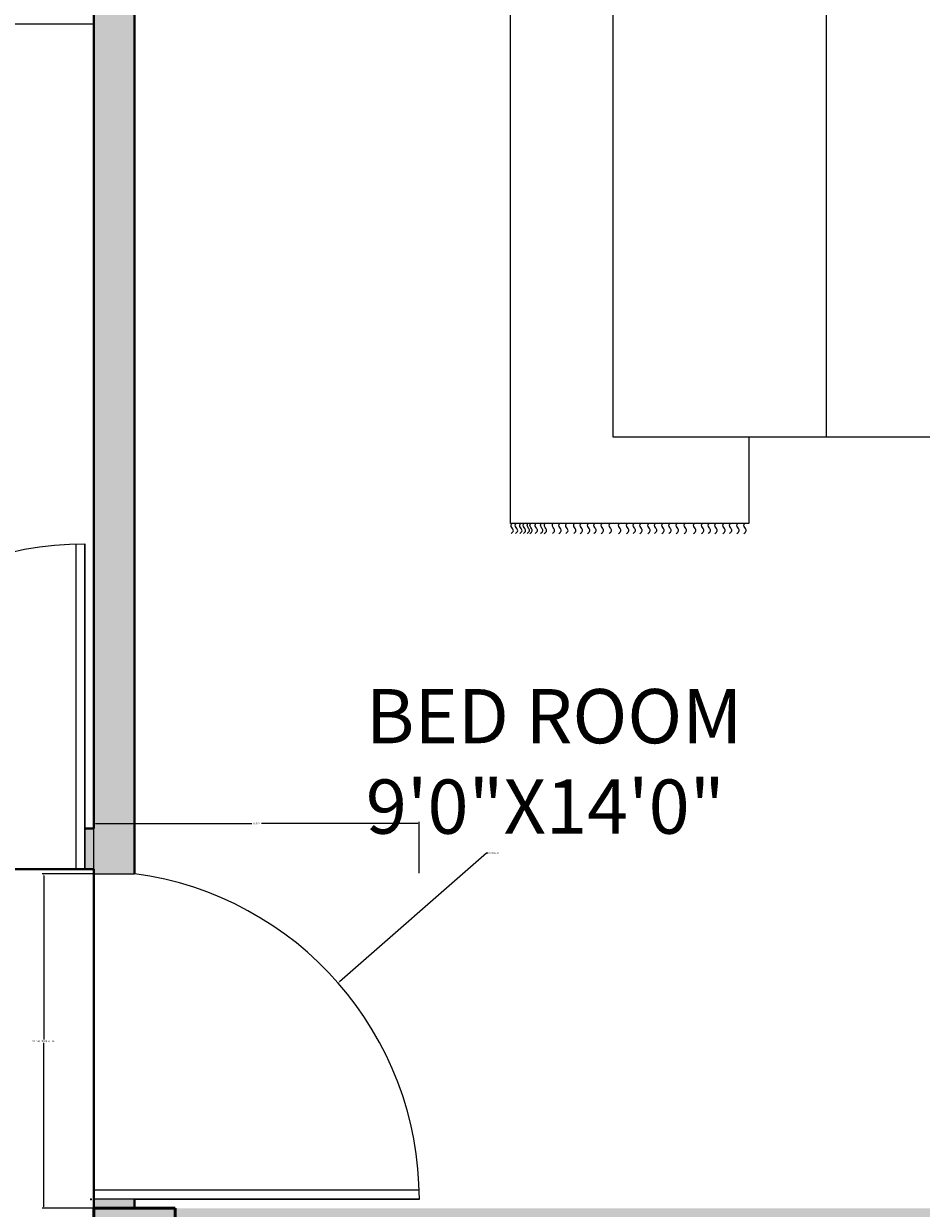
# Model space of a CAD drawing. Units: inches. Extents: x 25176543 to 25177243, y 80295576 to 80296086.
# Tile 8 of 11: x 25176997 to 25177096, y 80295848 to 80295979. Entities that reach past the tile are written whole.
import ezdxf

# ---------------------------------------------------------------- set-up
doc = ezdxf.new("R2010")
doc.units = ezdxf.units.IN
doc.header["$MEASUREMENT"] = 0
for name, color, linetype, lineweight in [('A-ANNO-DIMS', 2, 'Continuous', 18), ('A-AREA-IDEN', 7, 'Continuous', 18), ('A-COLS', 7, 'Continuous', 50), ('A-COLS-PATT', 251, 'Continuous', 13), ('A-DOOR', 3, 'Continuous', 25), ('A-FLOR-CASE', 8, 'Continuous', 25), ('A-WALL', 7, 'Continuous', 40), ('A-WALL-PATT', 146, 'Continuous', 13), ('furniture', 31, 'Continuous', 13)]:
    doc.layers.add(name, color=color, linetype=linetype, lineweight=lineweight)
doc.styles.get("Standard").update_dxf_attribs({"font": 'arial.ttf'})
doc.dimstyles.get("Standard").update_dxf_attribs({"dimtxt": 0.18, "dimasz": 0.18, "dimexe": 0.18, "dimexo": 0.0625, "dimgap": 0.09, "dimtad": 0, "dimtih": 1, "dimtoh": 1, "dimdec": 4, "dimzin": 0, "dimdsep": 46, "dimtxsty": 'Standard', "dimcen": 0.09, "dimadec": 0, "dimazin": 0, "dimtfac": 1, "dimtdec": 4, "dimtofl": 0, "dimtmove": 0, "dimatfit": 3, "dimfxl": 1, "dimtolj": 1, "dimtzin": 0, "dimarcsym": 0})

# ---------------------------------------------------------------- blocks, each defined once
blk = doc.blocks.new('BED-DOUBLE-WITH-NIGHTSTANDS')
for p, q in [((5.6, 61.62), (5.6, 51.56)), ((63.65, 61.72), (63.65, 51.66)), ((10.63, 56.59), (0.57, 56.59)), ((68.68, 56.69), (58.62, 56.69)), ((49.39, 52.82), (10.63, 52.82)), ((49.39, 52.82), (58, 46.47)), ((49.44, 52.82), (49.44, 46.47)), ((49.44, 52), (10.63, 52)), ((49.44, 46.47), (58, 46.47)), ((58.05, 34.96), (10.63, 34.96)), ((4.35, 0), (4.35, 26.37)), ((4.35, 26.37), (10.65, 26.37)), ((58.05, 26.37), (67.59, 26.37)), ((67.59, 26.37), (67.59, 0)), ((67.59, 0), (4.35, 0))]:
    blk.add_line(p, q)
for points in [[(0, 50.39), (10.63, 50.5), (10.63, 62.68), (0, 62.58)], [(58.05, 62.68), (58.05, 11.37), (10.63, 11.37), (10.63, 62.68)], [(58.05, 50.5), (68.68, 50.6), (68.68, 62.78), (58.05, 62.68)], [(29.88, 59.98), (29.88, 52.82), (15.98, 52.82), (15.98, 59.98)], [(49.44, 59.98), (49.44, 52.82), (35.55, 52.82), (35.55, 59.98)]]:
    blk.add_lwpolyline(points, close=True)
for centre in [(5.6, 56.59), (63.65, 56.69)]:
    blk.add_circle(centre, 3.92)
for points, knots in [([(3.23, 25.84), (3.32, 25.96), (3.52, 26.2), (3.86, 25.96), (4.14, 25.78), (4.29, 25.89), (4.35, 25.94)], [0, 0, 0, 0, 0.400747, 0.791423, 1.067667, 1.29709, 1.29709, 1.29709, 1.29709]), ([(3.23, 25.06), (3.32, 25.18), (3.52, 25.42), (3.86, 25.18), (4.14, 25.01), (4.29, 25.11), (4.35, 25.16)], [0, 0, 0, 0, 0.400747, 0.791423, 1.067667, 1.29709, 1.29709, 1.29709, 1.29709]), ([(68.71, 25.84), (68.61, 25.96), (68.42, 26.2), (68.08, 25.96), (67.8, 25.78), (67.65, 25.89), (67.58, 25.94)], [0, 0, 0, 0, 0.400747, 0.791423, 1.067667, 1.29709, 1.29709, 1.29709, 1.29709]), ([(68.71, 25.06), (68.61, 25.18), (68.42, 25.42), (68.08, 25.18), (67.8, 25.01), (67.65, 25.11), (67.58, 25.16)], [0, 0, 0, 0, 0.400747, 0.791423, 1.067667, 1.29709, 1.29709, 1.29709, 1.29709]), ([(3.23, 24.24), (3.32, 24.36), (3.52, 24.6), (3.86, 24.36), (4.14, 24.19), (4.29, 24.3), (4.35, 24.34)], [0, 0, 0, 0, 0.400747, 0.791423, 1.067667, 1.29709, 1.29709, 1.29709, 1.29709]), ([(3.23, 23.51), (3.32, 23.63), (3.52, 23.87), (3.86, 23.63), (4.14, 23.46), (4.29, 23.57), (4.35, 23.62)], [0, 0, 0, 0, 0.400747, 0.791423, 1.067667, 1.29709, 1.29709, 1.29709, 1.29709]), ([(68.71, 24.24), (68.61, 24.36), (68.42, 24.6), (68.08, 24.36), (67.8, 24.19), (67.65, 24.3), (67.58, 24.34)], [0, 0, 0, 0, 0.400747, 0.791423, 1.067667, 1.29709, 1.29709, 1.29709, 1.29709]), ([(68.71, 23.51), (68.61, 23.63), (68.42, 23.87), (68.08, 23.63), (67.8, 23.46), (67.65, 23.57), (67.58, 23.62)], [0, 0, 0, 0, 0.400747, 0.791423, 1.067667, 1.29709, 1.29709, 1.29709, 1.29709]), ([(3.23, 22.63), (3.32, 22.75), (3.52, 22.99), (3.86, 22.75), (4.14, 22.58), (4.29, 22.69), (4.35, 22.73)], [0, 0, 0, 0, 0.400747, 0.791423, 1.067667, 1.29709, 1.29709, 1.29709, 1.29709]), ([(68.71, 22.63), (68.61, 22.75), (68.42, 22.99), (68.08, 22.75), (67.8, 22.58), (67.65, 22.69), (67.58, 22.73)], [0, 0, 0, 0, 0.400747, 0.791423, 1.067667, 1.29709, 1.29709, 1.29709, 1.29709]), ([(3.23, 21.88), (3.32, 22), (3.52, 22.24), (3.86, 22), (4.14, 21.83), (4.29, 21.93), (4.35, 21.98)], [0, 0, 0, 0, 0.400747, 0.791423, 1.067667, 1.29709, 1.29709, 1.29709, 1.29709]), ([(3.23, 21.15), (3.32, 21.27), (3.52, 21.51), (3.86, 21.27), (4.14, 21.1), (4.29, 21.21), (4.35, 21.25)], [0, 0, 0, 0, 0.400747, 0.791423, 1.067667, 1.29709, 1.29709, 1.29709, 1.29709]), ([(68.71, 21.88), (68.61, 22), (68.42, 22.24), (68.08, 22), (67.8, 21.83), (67.65, 21.93), (67.58, 21.98)], [0, 0, 0, 0, 0.400747, 0.791423, 1.067667, 1.29709, 1.29709, 1.29709, 1.29709]), ([(68.71, 21.15), (68.61, 21.27), (68.42, 21.51), (68.08, 21.27), (67.8, 21.1), (67.65, 21.21), (67.58, 21.25)], [0, 0, 0, 0, 0.400747, 0.791423, 1.067667, 1.29709, 1.29709, 1.29709, 1.29709]), ([(3.23, 20.27), (3.32, 20.39), (3.52, 20.63), (3.86, 20.39), (4.14, 20.22), (4.29, 20.32), (4.35, 20.37)], [0, 0, 0, 0, 0.400747, 0.791423, 1.067667, 1.29709, 1.29709, 1.29709, 1.29709]), ([(68.71, 20.27), (68.61, 20.39), (68.42, 20.63), (68.08, 20.39), (67.8, 20.22), (67.65, 20.32), (67.58, 20.37)], [0, 0, 0, 0, 0.400747, 0.791423, 1.067667, 1.29709, 1.29709, 1.29709, 1.29709]), ([(3.23, 19.23), (3.32, 19.35), (3.52, 19.59), (3.86, 19.35), (4.14, 19.18), (4.29, 19.29), (4.35, 19.33)], [0, 0, 0, 0, 0.400747, 0.791423, 1.067667, 1.29709, 1.29709, 1.29709, 1.29709]), ([(3.23, 18.35), (3.32, 18.47), (3.52, 18.71), (3.86, 18.47), (4.14, 18.3), (4.29, 18.4), (4.35, 18.45)], [0, 0, 0, 0, 0.400747, 0.791423, 1.067667, 1.29709, 1.29709, 1.29709, 1.29709]), ([(68.71, 19.23), (68.61, 19.35), (68.42, 19.59), (68.08, 19.35), (67.8, 19.18), (67.65, 19.29), (67.58, 19.33)], [0, 0, 0, 0, 0.400747, 0.791423, 1.067667, 1.29709, 1.29709, 1.29709, 1.29709]), ([(68.71, 18.35), (68.61, 18.47), (68.42, 18.71), (68.08, 18.47), (67.8, 18.3), (67.65, 18.4), (67.58, 18.45)], [0, 0, 0, 0, 0.400747, 0.791423, 1.067667, 1.29709, 1.29709, 1.29709, 1.29709]), ([(3.23, 17.53), (3.32, 17.65), (3.52, 17.89), (3.86, 17.65), (4.14, 17.48), (4.29, 17.59), (4.35, 17.64)], [0, 0, 0, 0, 0.400747, 0.791423, 1.067667, 1.29709, 1.29709, 1.29709, 1.29709]), ([(68.71, 17.53), (68.61, 17.65), (68.42, 17.89), (68.08, 17.65), (67.8, 17.48), (67.65, 17.59), (67.58, 17.64)], [0, 0, 0, 0, 0.400747, 0.791423, 1.067667, 1.29709, 1.29709, 1.29709, 1.29709]), ([(3.23, 16.76), (3.32, 16.88), (3.52, 17.12), (3.86, 16.88), (4.14, 16.7), (4.29, 16.81), (4.35, 16.86)], [0, 0, 0, 0, 0.400747, 0.791423, 1.067667, 1.29709, 1.29709, 1.29709, 1.29709]), ([(3.23, 15.94), (3.32, 16.06), (3.52, 16.3), (3.86, 16.06), (4.14, 15.89), (4.29, 16), (4.35, 16.04)], [0, 0, 0, 0, 0.400747, 0.791423, 1.067667, 1.29709, 1.29709, 1.29709, 1.29709]), ([(68.71, 16.76), (68.61, 16.88), (68.42, 17.12), (68.08, 16.88), (67.8, 16.7), (67.65, 16.81), (67.58, 16.86)], [0, 0, 0, 0, 0.400747, 0.791423, 1.067667, 1.29709, 1.29709, 1.29709, 1.29709]), ([(68.71, 15.94), (68.61, 16.06), (68.42, 16.3), (68.08, 16.06), (67.8, 15.89), (67.65, 16), (67.58, 16.04)], [0, 0, 0, 0, 0.400747, 0.791423, 1.067667, 1.29709, 1.29709, 1.29709, 1.29709]), ([(3.23, 15.21), (3.32, 15.33), (3.52, 15.57), (3.86, 15.33), (4.14, 15.16), (4.29, 15.27), (4.35, 15.32)], [0, 0, 0, 0, 0.400747, 0.791423, 1.067667, 1.29709, 1.29709, 1.29709, 1.29709]), ([(3.23, 14.33), (3.32, 14.45), (3.52, 14.69), (3.86, 14.45), (4.14, 14.28), (4.29, 14.38), (4.35, 14.43)], [0, 0, 0, 0, 0.400747, 0.791423, 1.067667, 1.29709, 1.29709, 1.29709, 1.29709]), ([(68.71, 15.21), (68.61, 15.33), (68.42, 15.57), (68.08, 15.33), (67.8, 15.16), (67.65, 15.27), (67.58, 15.32)], [0, 0, 0, 0, 0.400747, 0.791423, 1.067667, 1.29709, 1.29709, 1.29709, 1.29709]), ([(68.71, 14.33), (68.61, 14.45), (68.42, 14.69), (68.08, 14.45), (67.8, 14.28), (67.65, 14.38), (67.58, 14.43)], [0, 0, 0, 0, 0.400747, 0.791423, 1.067667, 1.29709, 1.29709, 1.29709, 1.29709]), ([(3.23, 13.58), (3.32, 13.7), (3.52, 13.94), (3.86, 13.7), (4.14, 13.53), (4.29, 13.63), (4.35, 13.68)], [0, 0, 0, 0, 0.400747, 0.791423, 1.067667, 1.29709, 1.29709, 1.29709, 1.29709]), ([(3.23, 12.85), (3.32, 12.97), (3.52, 13.21), (3.86, 12.97), (4.14, 12.8), (4.29, 12.9), (4.35, 12.95)], [0, 0, 0, 0, 0.400747, 0.791423, 1.067667, 1.29709, 1.29709, 1.29709, 1.29709]), ([(68.71, 13.58), (68.61, 13.7), (68.42, 13.94), (68.08, 13.7), (67.8, 13.53), (67.65, 13.63), (67.58, 13.68)], [0, 0, 0, 0, 0.400747, 0.791423, 1.067667, 1.29709, 1.29709, 1.29709, 1.29709]), ([(68.71, 12.85), (68.61, 12.97), (68.42, 13.21), (68.08, 12.97), (67.8, 12.8), (67.65, 12.9), (67.58, 12.95)], [0, 0, 0, 0, 0.400747, 0.791423, 1.067667, 1.29709, 1.29709, 1.29709, 1.29709]), ([(3.23, 11.97), (3.32, 12.09), (3.52, 12.33), (3.86, 12.09), (4.14, 11.92), (4.29, 12.02), (4.35, 12.07)], [0, 0, 0, 0, 0.400747, 0.791423, 1.067667, 1.29709, 1.29709, 1.29709, 1.29709]), ([(68.71, 11.97), (68.61, 12.09), (68.42, 12.33), (68.08, 12.09), (67.8, 11.92), (67.65, 12.02), (67.58, 12.07)], [0, 0, 0, 0, 0.400747, 0.791423, 1.067667, 1.29709, 1.29709, 1.29709, 1.29709]), ([(3.23, 10.93), (3.32, 11.05), (3.52, 11.29), (3.86, 11.05), (4.14, 10.88), (4.29, 10.99), (4.35, 11.03)], [0, 0, 0, 0, 0.400747, 0.791423, 1.067667, 1.29709, 1.29709, 1.29709, 1.29709]), ([(68.71, 10.93), (68.61, 11.05), (68.42, 11.29), (68.08, 11.05), (67.8, 10.88), (67.65, 10.99), (67.58, 11.03)], [0, 0, 0, 0, 0.400747, 0.791423, 1.067667, 1.29709, 1.29709, 1.29709, 1.29709]), ([(3.23, 10.05), (3.32, 10.17), (3.52, 10.41), (3.86, 10.17), (4.14, 10), (4.29, 10.1), (4.35, 10.15)], [0, 0, 0, 0, 0.400747, 0.791423, 1.067667, 1.29709, 1.29709, 1.29709, 1.29709]), ([(3.23, 9.23), (3.32, 9.35), (3.52, 9.59), (3.86, 9.35), (4.14, 9.18), (4.29, 9.29), (4.35, 9.34)], [0, 0, 0, 0, 0.400747, 0.791423, 1.067667, 1.29709, 1.29709, 1.29709, 1.29709]), ([(68.71, 10.05), (68.61, 10.17), (68.42, 10.41), (68.08, 10.17), (67.8, 10), (67.65, 10.1), (67.58, 10.15)], [0, 0, 0, 0, 0.400747, 0.791423, 1.067667, 1.29709, 1.29709, 1.29709, 1.29709]), ([(68.71, 9.23), (68.61, 9.35), (68.42, 9.59), (68.08, 9.35), (67.8, 9.18), (67.65, 9.29), (67.58, 9.34)], [0, 0, 0, 0, 0.400747, 0.791423, 1.067667, 1.29709, 1.29709, 1.29709, 1.29709]), ([(3.23, 8.54), (3.32, 8.66), (3.52, 8.9), (3.86, 8.66), (4.14, 8.49), (4.29, 8.6), (4.35, 8.65)], [0, 0, 0, 0, 0.400747, 0.791423, 1.067667, 1.29709, 1.29709, 1.29709, 1.29709]), ([(3.23, 7.73), (3.32, 7.85), (3.52, 8.09), (3.86, 7.85), (4.14, 7.68), (4.29, 7.78), (4.35, 7.83)], [0, 0, 0, 0, 0.400747, 0.791423, 1.067667, 1.29709, 1.29709, 1.29709, 1.29709]), ([(68.71, 8.54), (68.61, 8.66), (68.42, 8.9), (68.08, 8.66), (67.8, 8.49), (67.65, 8.6), (67.58, 8.65)], [0, 0, 0, 0, 0.400747, 0.791423, 1.067667, 1.29709, 1.29709, 1.29709, 1.29709]), ([(68.71, 7.73), (68.61, 7.85), (68.42, 8.09), (68.08, 7.85), (67.8, 7.68), (67.65, 7.78), (67.58, 7.83)], [0, 0, 0, 0, 0.400747, 0.791423, 1.067667, 1.29709, 1.29709, 1.29709, 1.29709]), ([(3.23, 7), (3.32, 7.12), (3.52, 7.36), (3.86, 7.12), (4.14, 6.95), (4.29, 7.05), (4.35, 7.1)], [0, 0, 0, 0, 0.400747, 0.791423, 1.067667, 1.29709, 1.29709, 1.29709, 1.29709]), ([(68.71, 7), (68.61, 7.12), (68.42, 7.36), (68.08, 7.12), (67.8, 6.95), (67.65, 7.05), (67.58, 7.1)], [0, 0, 0, 0, 0.400747, 0.791423, 1.067667, 1.29709, 1.29709, 1.29709, 1.29709]), ([(3.23, 6.12), (3.32, 6.24), (3.52, 6.48), (3.86, 6.24), (4.14, 6.07), (4.29, 6.17), (4.35, 6.22)], [0, 0, 0, 0, 0.400747, 0.791423, 1.067667, 1.29709, 1.29709, 1.29709, 1.29709]), ([(3.23, 5.36), (3.32, 5.49), (3.52, 5.73), (3.86, 5.49), (4.14, 5.31), (4.29, 5.42), (4.35, 5.47)], [0, 0, 0, 0, 0.400747, 0.791423, 1.067667, 1.29709, 1.29709, 1.29709, 1.29709]), ([(68.71, 6.12), (68.61, 6.24), (68.42, 6.48), (68.08, 6.24), (67.8, 6.07), (67.65, 6.17), (67.58, 6.22)], [0, 0, 0, 0, 0.400747, 0.791423, 1.067667, 1.29709, 1.29709, 1.29709, 1.29709]), ([(68.71, 5.36), (68.61, 5.49), (68.42, 5.73), (68.08, 5.49), (67.8, 5.31), (67.65, 5.42), (67.58, 5.47)], [0, 0, 0, 0, 0.400747, 0.791423, 1.067667, 1.29709, 1.29709, 1.29709, 1.29709]), ([(3.23, 4.64), (3.32, 4.76), (3.52, 5), (3.86, 4.76), (4.14, 4.59), (4.29, 4.69), (4.35, 4.74)], [0, 0, 0, 0, 0.400747, 0.791423, 1.067667, 1.29709, 1.29709, 1.29709, 1.29709]), ([(3.23, 3.75), (3.32, 3.88), (3.52, 4.12), (3.86, 3.88), (4.14, 3.7), (4.29, 3.81), (4.35, 3.86)], [0, 0, 0, 0, 0.400747, 0.791423, 1.067667, 1.29709, 1.29709, 1.29709, 1.29709]), ([(68.71, 4.64), (68.61, 4.76), (68.42, 5), (68.08, 4.76), (67.8, 4.59), (67.66, 4.69), (67.59, 4.73)], [0, 0, 0, 0, 0.400747, 0.791423, 1.067667, 1.283686, 1.283686, 1.283686, 1.283686]), ([(68.71, 3.75), (68.61, 3.88), (68.42, 4.11), (68.08, 3.88), (67.8, 3.7), (67.66, 3.81), (67.59, 3.85)], [0, 0, 0, 0, 0.400747, 0.791423, 1.067667, 1.283686, 1.283686, 1.283686, 1.283686]), ([(3.23, 3.33), (3.32, 3.45), (3.52, 3.7), (3.86, 3.44), (4.14, 3.27), (4.29, 3.38), (4.35, 3.43)], [0, 0, 0, 0, 0.407265, 0.802015, 1.07826, 1.307683, 1.307683, 1.307683, 1.307683]), ([(3.23, 2.76), (3.32, 2.88), (3.52, 3.12), (3.86, 2.88), (4.14, 2.71), (4.29, 2.81), (4.35, 2.86)], [0, 0, 0, 0, 0.400747, 0.791423, 1.067667, 1.29709, 1.29709, 1.29709, 1.29709]), ([(68.71, 3.33), (68.61, 3.45), (68.42, 3.69), (68.08, 3.45), (67.8, 3.27), (67.66, 3.38), (67.59, 3.42)], [0, 0, 0, 0, 0.402903, 0.794912, 1.071156, 1.287177, 1.287177, 1.287177, 1.287177]), ([(68.71, 2.73), (68.61, 2.85), (68.42, 3.09), (68.08, 2.85), (67.8, 2.68), (67.66, 2.78), (67.59, 2.82)], [0, 0, 0, 0, 0.400747, 0.791423, 1.067667, 1.283686, 1.283686, 1.283686, 1.283686]), ([(3.23, 2.18), (3.32, 2.31), (3.52, 2.55), (3.86, 2.31), (4.14, 2.13), (4.29, 2.24), (4.35, 2.29)], [0, 0, 0, 0, 0.400747, 0.791423, 1.067667, 1.29709, 1.29709, 1.29709, 1.29709]), ([(3.23, 1.88), (3.32, 2), (3.52, 2.24), (3.86, 2), (4.14, 1.82), (4.29, 1.93), (4.35, 1.98)], [0, 0, 0, 0, 0.400747, 0.791423, 1.067667, 1.29709, 1.29709, 1.29709, 1.29709]), ([(3.23, 1.46), (3.32, 1.58), (3.52, 1.82), (3.86, 1.58), (4.14, 1.41), (4.29, 1.51), (4.35, 1.56)], [0, 0, 0, 0, 0.400747, 0.791423, 1.067667, 1.29709, 1.29709, 1.29709, 1.29709]), ([(3.23, 1.06), (3.32, 1.18), (3.52, 1.42), (3.86, 1.18), (4.14, 1.01), (4.29, 1.11), (4.35, 1.16)], [0, 0, 0, 0, 0.400747, 0.791423, 1.067667, 1.29709, 1.29709, 1.29709, 1.29709]), ([(68.71, 1.43), (68.61, 1.55), (68.42, 1.79), (68.08, 1.55), (67.8, 1.38), (67.65, 1.48), (67.58, 1.53)], [0, 0, 0, 0, 0.400747, 0.791423, 1.067667, 1.29709, 1.29709, 1.29709, 1.29709]), ([(68.71, 2.16), (68.61, 2.28), (68.42, 2.52), (68.08, 2.28), (67.8, 2.11), (67.66, 2.21), (67.59, 2.25)], [0, 0, 0, 0, 0.400747, 0.791423, 1.067667, 1.283686, 1.283686, 1.283686, 1.283686]), ([(68.71, 1.85), (68.61, 1.97), (68.42, 2.21), (68.08, 1.97), (67.8, 1.8), (67.66, 1.9), (67.59, 1.94)], [0, 0, 0, 0, 0.400747, 0.791423, 1.067667, 1.283686, 1.283686, 1.283686, 1.283686]), ([(3.23, 0.57), (3.32, 0.7), (3.52, 0.94), (3.86, 0.7), (4.14, 0.52), (4.29, 0.63), (4.35, 0.68)], [0, 0, 0, 0, 0.400747, 0.791423, 1.067667, 1.29709, 1.29709, 1.29709, 1.29709]), ([(3.23, 0.07), (3.32, 0.19), (3.52, 0.43), (3.86, 0.19), (4.14, 0.02), (4.29, 0.13), (4.35, 0.18)], [0, 0, 0, 0, 0.400747, 0.791423, 1.067667, 1.29709, 1.29709, 1.29709, 1.29709]), ([(68.71, 1.03), (68.61, 1.15), (68.42, 1.39), (68.08, 1.15), (67.8, 0.98), (67.65, 1.09), (67.58, 1.13)], [0, 0, 0, 0, 0.400747, 0.791423, 1.067667, 1.29709, 1.29709, 1.29709, 1.29709]), ([(68.71, 0.55), (68.61, 0.67), (68.42, 0.91), (68.08, 0.67), (67.8, 0.49), (67.65, 0.6), (67.58, 0.65)], [0, 0, 0, 0, 0.400747, 0.791423, 1.067667, 1.29709, 1.29709, 1.29709, 1.29709]), ([(68.71, 0.07), (68.61, 0.19), (68.42, 0.43), (68.08, 0.19), (67.8, 0.02), (67.65, 0.13), (67.58, 0.18)], [0, 0, 0, 0, 0.400747, 0.791423, 1.067667, 1.29709, 1.29709, 1.29709, 1.29709])]:
    blk.add_open_spline(points, degree=3, knots=knots)
blk = doc.blocks.new('DOOR-36IN')
for p, q in [((36, 37), (31.5, 37)), ((36, 1), (36, 37)), ((0, 2), (36, 2)), ((36, 1), (0, 1)), ((0, 1), (36, 1)), ((36, 0), (36, 1))]:
    blk.add_line(p, q)
blk.add_arc((36.32, 1), 36.32, 97.6281, 180)
blk = doc.blocks.new('DOOR-36IN-OFFSET')
for p, q in [((0, 1), (0, 37)), ((0, 37), (4.5, 37)), ((36, 2), (0, 2)), ((0, 0), (0, 1)), ((4.5, 1), (0, 1)), ((4.5, 1), (36, 1)), ((36, 1), (4.5, 1))]:
    blk.add_line(p, q)
blk.add_arc((-0.32, 1), 36.32, 0, 82.3719)
blk = doc.blocks.new('COLUMN-9IN-SQ')
for p, q in [((9, 9), (0, 9)), ((0, 9), (0, 0)), ((9, 0), (9, 9)), ((0, 0), (9, 0))]:
    blk.add_line(p, q)
blk = doc.blocks.new('*D42')
at = {"layer": 'A-ANNO-DIMS', "color": 0, "lineweight": -2, "transparency": 16777216}
for p, q in [((25177004.24, 80295885.3), (25176998.57, 80295885.3)), ((25176998.75, 80295885.12), (25176998.75, 80295866.99)), ((25176998.75, 80295848.48), (25176998.75, 80295866.62)), ((25177004.24, 80295848.3), (25176998.57, 80295848.3))]:
    blk.add_line(p, q, dxfattribs=at)
at = {"layer": 'A-ANNO-DIMS', "color": 0, "transparency": 16777216}
for points in [[(25176998.72, 80295885.12), (25176998.78, 80295885.12), (25176998.75, 80295885.3)], [(25176998.72, 80295848.48), (25176998.78, 80295848.48), (25176998.75, 80295848.3)]]:
    blk.add_solid(points, dxfattribs=at)
at = {"layer": 'Defpoints', "color": 0, "transparency": 16777216}
for p in [(25176998.75, 80295885.3), (25177004.3, 80295885.3), (25177004.3, 80295848.3)]:
    blk.add_point(p, dxfattribs=at)
at = {"layer": 'A-ANNO-DIMS', "color": 0, "transparency": 16777216, "insert": (25176998.75, 80295866.8), "char_height": 0.18, "attachment_point": 5}
blk.add_mtext('\\A1;OFFSET DOOR 37 TYP.', dxfattribs=at)
blk = doc.blocks.new('*D43')
at = {"layer": 'A-ANNO-DIMS', "color": 0, "lineweight": -2, "transparency": 16777216}
for p, q in [((25177004.3, 80295885.36), (25177004.3, 80295891.03)), ((25177004.48, 80295890.85), (25177021.77, 80295890.85)), ((25177040.12, 80295890.85), (25177022.83, 80295890.85)), ((25177040.3, 80295885.36), (25177040.3, 80295891.03))]:
    blk.add_line(p, q, dxfattribs=at)
at = {"layer": 'A-ANNO-DIMS', "color": 0, "transparency": 16777216}
for points in [[(25177004.48, 80295890.88), (25177004.48, 80295890.82), (25177004.3, 80295890.85)], [(25177040.12, 80295890.88), (25177040.12, 80295890.82), (25177040.3, 80295890.85)]]:
    blk.add_solid(points, dxfattribs=at)
at = {"layer": 'Defpoints', "color": 0, "transparency": 16777216}
for p in [(25177040.3, 80295890.85), (25177004.3, 80295885.3), (25177040.3, 80295885.3)]:
    blk.add_point(p, dxfattribs=at)
at = {"layer": 'A-ANNO-DIMS', "color": 0, "transparency": 16777216, "insert": (25177022.3, 80295890.85), "char_height": 0.18, "attachment_point": 5}
blk.add_mtext('\\A1;36 TYP.', dxfattribs=at)
blk = doc.blocks.new('*D48')
at = {"layer": 'A-ANNO-DIMS', "color": 0, "lineweight": -2, "transparency": 16777216}
for p, q in [((25176625.3, 80295890.36), (25176625.3, 80296052.23)), ((25176625.48, 80296052.05), (25176875.16, 80296052.05)), ((25177125.62, 80296052.05), (25176875.95, 80296052.05)), ((25177125.8, 80296025.36), (25177125.8, 80296052.23))]:
    blk.add_line(p, q, dxfattribs=at)
at = {"layer": 'A-ANNO-DIMS', "color": 0, "transparency": 16777216}
for points in [[(25176625.48, 80296052.08), (25176625.48, 80296052.02), (25176625.3, 80296052.05)], [(25177125.62, 80296052.08), (25177125.62, 80296052.02), (25177125.8, 80296052.05)]]:
    blk.add_solid(points, dxfattribs=at)
at = {"layer": 'Defpoints', "color": 0, "transparency": 16777216}
for p in [(25177125.8, 80296052.05), (25177125.8, 80296025.3), (25176625.3, 80295890.3)]:
    blk.add_point(p, dxfattribs=at)
at = {"layer": 'A-ANNO-DIMS', "color": 0, "transparency": 16777216, "insert": (25176875.55, 80296052.05), "char_height": 0.18, "attachment_point": 5}
blk.add_mtext('\\A1;500.5', dxfattribs=at)
blk = doc.blocks.new('*D76')
at = {"layer": 'A-ANNO-DIMS', "color": 0, "lineweight": -2, "transparency": 16777216}
for p, q in [((25177047.72, 80295887.57), (25177031.45, 80295873.34)), ((25177047.9, 80295887.57), (25177047.72, 80295887.57)), ((25177003.89, 80295849.3), (25177004.07, 80295849.3)), ((25177003.98, 80295849.21), (25177003.98, 80295849.39))]:
    blk.add_line(p, q, dxfattribs=at)
at = {"layer": 'A-ANNO-DIMS', "color": 0, "transparency": 16777216}
blk.add_solid([(25177031.43, 80295873.36), (25177031.47, 80295873.32), (25177031.31, 80295873.22)], dxfattribs=at)
at = {"layer": 'Defpoints', "color": 0, "transparency": 16777216}
for p in [(25177031.31, 80295873.22), (25177003.98, 80295849.3)]:
    blk.add_point(p, dxfattribs=at)
at = {"layer": 'A-ANNO-DIMS', "color": 0, "transparency": 16777216, "insert": (25177048.57, 80295887.57), "char_height": 0.18, "attachment_point": 5}
blk.add_mtext('\\A1;2X R36.32', dxfattribs=at)

msp = doc.modelspace()

# ---------------------------------------------------------------- hatches: boundary and pattern name
at = {"layer": 'A-COLS-PATT'}
h = msp.add_hatch(color=256, dxfattribs=at)
h.dxf.hatch_style = 1
h.paths.add_polyline_path([(25176658.8016, 80296025.3022), (25176649.8016, 80296025.3022), (25176649.8016, 80296016.3022), (25176658.8016, 80296016.3022)])
h.paths.add_polyline_path([(25176819.3016, 80296025.3022), (25176810.3016, 80296025.3022), (25176810.3016, 80296016.3022), (25176819.3016, 80296016.3022)])
h.paths.add_polyline_path([(25176876.3016, 80296025.3022), (25176867.3016, 80296025.3022), (25176867.3016, 80296016.3022), (25176876.3016, 80296016.3022)])
h.paths.add_polyline_path([(25177013.3016, 80296025.3022), (25177004.3016, 80296025.3022), (25177004.3016, 80296016.3022), (25177013.3016, 80296016.3022)])
h.paths.add_polyline_path([(25176819.3016, 80295890.3022), (25176810.3016, 80295890.3022), (25176810.3016, 80295881.3022), (25176819.3016, 80295881.3022)])
h.paths.add_polyline_path([(25176658.8016, 80295890.3022), (25176649.8016, 80295890.3022), (25176649.8016, 80295881.3022), (25176658.8016, 80295881.3022)])
h.paths.add_polyline_path([(25177125.8016, 80296025.3022), (25177116.8016, 80296025.3022), (25177116.8016, 80296016.3022), (25177125.8016, 80296016.3022)])
h.paths.add_polyline_path([(25177125.8016, 80295848.3022), (25177116.8016, 80295848.3022), (25177116.8016, 80295839.3022), (25177125.8016, 80295839.3022)])
h.paths.add_polyline_path([(25177013.3016, 80295848.3022), (25177004.3016, 80295848.3022), (25177004.3016, 80295839.3022), (25177013.3016, 80295839.3022)])
h.paths.add_polyline_path([(25177125.8016, 80295676.8022), (25177116.8016, 80295676.8022), (25177116.8016, 80295667.8022), (25177125.8016, 80295667.8022)])
h.paths.add_polyline_path([(25177013.3016, 80295676.8022), (25177004.3016, 80295676.8022), (25177004.3016, 80295667.8022), (25177013.3016, 80295667.8022)])
h.paths.add_polyline_path([(25176842.3016, 80295676.8022), (25176833.3016, 80295676.8022), (25176833.3016, 80295667.8022), (25176842.3016, 80295667.8022)])
h.paths.add_polyline_path([(25176893.3016, 80295676.8022), (25176884.3016, 80295676.8022), (25176884.3016, 80295667.8022), (25176893.3016, 80295667.8022)])
h.paths.add_polyline_path([(25176842.3016, 80295807.3022), (25176833.3016, 80295807.3022), (25176833.3016, 80295798.3022), (25176842.3016, 80295798.3022)])
h.paths.add_polyline_path([(25176658.8016, 80295807.3022), (25176649.8016, 80295807.3022), (25176649.8016, 80295798.3022), (25176658.8016, 80295798.3022)])
h.paths.add_polyline_path([(25176658.8016, 80295676.8022), (25176649.8016, 80295676.8022), (25176649.8016, 80295667.8022), (25176658.8016, 80295667.8022)])
at = {"layer": 'A-WALL-PATT'}
h = msp.add_hatch(color=256, dxfattribs=at)
h.dxf.hatch_style = 1
h.paths.add_polyline_path([(25176695.189, 80296025.3022), (25176658.8016, 80296025.3022), (25176658.8016, 80296016.3022), (25176695.189, 80296016.3022)])
h.paths.add_polyline_path([(25176810.3016, 80296025.3022), (25176755.189, 80296025.3022), (25176755.189, 80296016.3022), (25176810.3016, 80296016.3022)])
h.paths.add_polyline_path([(25176819.3016, 80296016.3022), (25176814.8016, 80296016.3022), (25176814.8016, 80295965.3022), (25176819.3016, 80295965.3022)], flags=17)
h.paths.add_polyline_path([(25176828.0421, 80296025.3022), (25176819.3016, 80296025.3022), (25176819.3016, 80296016.3022), (25176828.0421, 80296016.3022)])
h.paths.add_polyline_path([(25176867.3016, 80296025.3022), (25176852.0421, 80296025.3022), (25176852.0421, 80296016.3022), (25176867.3016, 80296016.3022)])
h.paths.add_polyline_path([(25176885.1873, 80296025.3022), (25176876.3016, 80296025.3022), (25176876.3016, 80296016.3022), (25176885.1873, 80296016.3022)])
h.paths.add_polyline_path([(25176919.8016, 80296025.3022), (25176909.1873, 80296025.3022), (25176909.1873, 80296016.3022), (25176919.8016, 80296016.3022)])
h.paths.add_polyline_path([(25176924.3016, 80296016.3022), (25176919.8016, 80296016.3022), (25176919.8016, 80295890.3022), (25176904.8016, 80295890.3022), (25176904.8016, 80295885.8022), (25176967.3016, 80295885.8022), (25176967.3016, 80295890.3022), (25176924.3016, 80295890.3022)])
h.paths.add_polyline_path([(25176924.3016, 80296025.3022), (25176919.8016, 80296025.3022), (25176919.8016, 80296016.3022), (25176924.3016, 80296016.3022)])
h.paths.add_polyline_path([(25176938.7147, 80296025.3022), (25176924.3016, 80296025.3022), (25176924.3016, 80296016.3022), (25176938.7147, 80296016.3022)])
h.paths.add_polyline_path([(25176871.8016, 80296016.3022), (25176867.3016, 80296016.3022), (25176867.3016, 80295932.3022), (25176819.3016, 80295932.3022), (25176819.3016, 80295933.3022), (25176814.8016, 80295933.3022), (25176814.8016, 80295932.3022), (25176814.8016, 80295927.3022), (25176819.3016, 80295927.3022), (25176819.3016, 80295927.8022), (25176867.3016, 80295927.8022), (25176867.3016, 80295885.8022), (25176871.8016, 80295885.8022), (25176872.8016, 80295885.8022), (25176872.8016, 80295890.3022), (25176871.8016, 80295890.3022)])
h.paths.add_polyline_path([(25177004.3016, 80296025.3022), (25176986.7147, 80296025.3022), (25176986.7147, 80296016.3022), (25177004.3016, 80296016.3022)])
h.paths.add_polyline_path([(25177035.845, 80296025.3022), (25177013.3016, 80296025.3022), (25177013.3016, 80296016.3022), (25177035.845, 80296016.3022)])
h.paths.add_polyline_path([(25177008.8016, 80296016.3022), (25177004.3016, 80296016.3022), (25177004.3016, 80295890.3022), (25177003.3016, 80295890.3022), (25177003.3016, 80295885.8022), (25177004.3016, 80295885.8022), (25177004.3016, 80295885.3022), (25177008.8016, 80295885.3022)])
h.paths.add_polyline_path([(25177116.8016, 80296025.3022), (25177095.845, 80296025.3022), (25177095.845, 80296016.3022), (25177116.8016, 80296016.3022)])
h.paths.add_polyline_path([(25177125.8016, 80296016.3022), (25177116.8016, 80296016.3022), (25177116.8016, 80295971.1334), (25177121.3016, 80295971.1334), (25177125.8016, 80295971.1334)])
h.paths.add_polyline_path([(25177116.8016, 80295848.3022), (25177013.3016, 80295848.3022), (25177013.3016, 80295843.8022), (25177116.8016, 80295843.8022)])
h.paths.add_polyline_path([(25177125.8016, 80295911.1334), (25177116.8016, 80295911.1334), (25177116.8016, 80295848.3022), (25177125.8016, 80295848.3022)])
h.paths.add_polyline_path([(25177008.8016, 80295802.3022), (25177004.3016, 80295802.3022), (25177004.3016, 80295676.8022), (25177008.8016, 80295676.8022)])
h.paths.add_polyline_path([(25176658.8016, 80295705.5694), (25176649.8016, 80295705.5694), (25176649.8016, 80295676.8022), (25176658.8016, 80295676.8022)])
h.paths.add_polyline_path([(25176658.8016, 80295798.3022), (25176649.8016, 80295798.3022), (25176649.8016, 80295765.5694), (25176654.3016, 80295765.5694), (25176658.8016, 80295765.5694)])
h.paths.add_polyline_path([(25176833.3016, 80295807.3022), (25176658.8016, 80295807.3022), (25176658.8016, 80295802.8022), (25176833.3016, 80295802.8022)])
h.paths.add_polyline_path([(25176842.3016, 80295761.3022), (25176837.8016, 80295761.3022), (25176837.8016, 80295676.8022), (25176842.3016, 80295676.8022)])
h.paths.add_polyline_path([(25176649.8016, 80295807.3022), (25176629.8016, 80295807.3022), (25176629.8016, 80295885.8022), (25176649.8016, 80295885.8022), (25176649.8016, 80295890.3022), (25176625.3016, 80295890.3022), (25176625.3016, 80295802.8022), (25176649.8016, 80295802.8022)])
h.paths.add_polyline_path([(25176810.3016, 80295890.3022), (25176658.8016, 80295890.3022), (25176658.8016, 80295885.8022), (25176810.3016, 80295885.8022)])
h.paths.add_polyline_path([(25176658.8016, 80295922.9263), (25176649.8016, 80295922.9263), (25176649.8016, 80295890.3022), (25176658.8016, 80295890.3022)])
h.paths.add_polyline_path([(25176658.8016, 80296016.3022), (25176649.8016, 80296016.3022), (25176649.8016, 80295982.9263), (25176654.3016, 80295982.9263), (25176658.8016, 80295982.9263)])
h = msp.add_hatch(color=256, dxfattribs=at)
h.dxf.hatch_style = 1
h.paths.add_polyline_path([(25177008.8016, 80295839.3022), (25177004.3016, 80295839.3022), (25177004.3016, 80295838.3022), (25177008.8016, 80295838.3022)])
h.paths.add_polyline_path([(25177008.8016, 80295849.3022), (25177004.3016, 80295849.3022), (25177004.3016, 80295848.3022), (25177008.8016, 80295848.3022)])

# ---------------------------------------------------------------- linework, layer by layer
at = {"layer": 'A-FLOR-CASE'}
msp.add_line((25176951.2221, 80295979.3235), (25177004.3016, 80295979.3235), dxfattribs=at)
at = {"layer": 'A-WALL'}
for p, q in [((25177004.3016, 80296025.3022), (25177004.3016, 80295890.3022)), ((25177008.8016, 80296016.3022), (25177008.8016, 80295885.3022)), ((25177003.3016, 80295890.3022), (25177004.3016, 80295890.3022)), ((25176867.3016, 80295885.8022), (25177004.3016, 80295885.8022)), ((25177004.3016, 80295885.8022), (25177004.3016, 80295667.8022)), ((25177008.8016, 80295849.3022), (25177008.8016, 80295848.3022))]:
    msp.add_line(p, q, dxfattribs=at)

# ---------------------------------------------------------------- block references
at = {"layer": 'A-COLS', "rotation": 90.0000001422956}
msp.add_blockref('COLUMN-9IN-SQ', (25177013.3018, 80295839.3026), dxfattribs=at)
at = {"layer": 'A-DOOR', "extrusion": (0, 0, -1), "zscale": -1, "rotation": 270.0000000097776}
msp.add_blockref('DOOR-36IN', (-25177004.3018, 80295921.8018), dxfattribs=at)
at = {"layer": 'A-DOOR'}
msp.add_blockref('DOOR-36IN-OFFSET', (25177004.302, 80295848.302), dxfattribs=at)
at = {"layer": 'furniture', "rotation": 269.9999999743436}
msp.add_blockref('BED-DOUBLE-WITH-NIGHTSTANDS', (25177050.3784, 80295991.6444), dxfattribs=at)

# ---------------------------------------------------------------- texts
at = {"layer": 'A-AREA-IDEN', "insert": (25177034.3813, 80295905.7333), "char_height": 6, "attachment_point": 1}
msp.add_mtext_dynamic_manual_height_columns('BED ROOM\\P9\'0"X14\'0"', width=53.227943, gutter_width=1, heights=[0], dxfattribs=at)

# ---------------------------------------------------------------- dimensions: what is measured, and where the dimension line sits
at = {"layer": 'A-ANNO-DIMS'}
dim = msp.add_linear_dim(base=(25177125.8016, 80296052.0522), p1=(25176625.3016, 80295890.3022), p2=(25177125.8016, 80296025.3022), dimstyle='Standard', override={"dimdec": 1, "dimlfac": 1, "dimrnd": 0, "dimzin": 0, "dimdsep": 46, "dimlunit": 2}, dxfattribs=at)
dim.commit()
dim.dimension.update_dxf_attribs({"geometry": '*D48', "text_midpoint": (25176875.5516, 80296052.0522)})
dim = msp.add_linear_dim(base=(25177040.3016, 80295890.8522), p1=(25177004.3016, 80295885.3022), p2=(25177040.3016, 80295885.3022), text='<> TYP.', dimstyle='Standard', override={"dimdec": 0, "dimlfac": 1, "dimrnd": 0, "dimzin": 0, "dimdsep": 46, "dimlunit": 2}, dxfattribs=at)
dim.commit()
dim.dimension.update_dxf_attribs({"geometry": '*D43', "text_midpoint": (25177022.3016, 80295890.8522)})
dim = msp.add_radius_dim(center=(25177003.9801, 80295849.3022), mpoint=(25177031.3149, 80295873.2199), text='2X <>', dimstyle='Standard', override={"dimdec": 2, "dimlfac": 1, "dimrnd": 0, "dimzin": 0, "dimdsep": 46, "dimlunit": 2}, dxfattribs=at)
dim.commit()
dim.dimension.update_dxf_attribs({"geometry": '*D76', "text_midpoint": (25177048.5696, 80295887.5705), "dimtype": 164})
dim = msp.add_linear_dim(base=(25176998.7516, 80295885.3022), p1=(25177004.3016, 80295848.3022), p2=(25177004.3016, 80295885.3022), angle=90, text='OFFSET DOOR <> TYP.', dimstyle='Standard', override={"dimdec": 0, "dimlfac": 1, "dimrnd": 0, "dimzin": 0, "dimdsep": 46, "dimlunit": 2}, dxfattribs=at)
dim.commit()
dim.dimension.update_dxf_attribs({"geometry": '*D42', "text_midpoint": (25176998.7516, 80295866.8022)})

doc.saveas('drawing.dxf')
